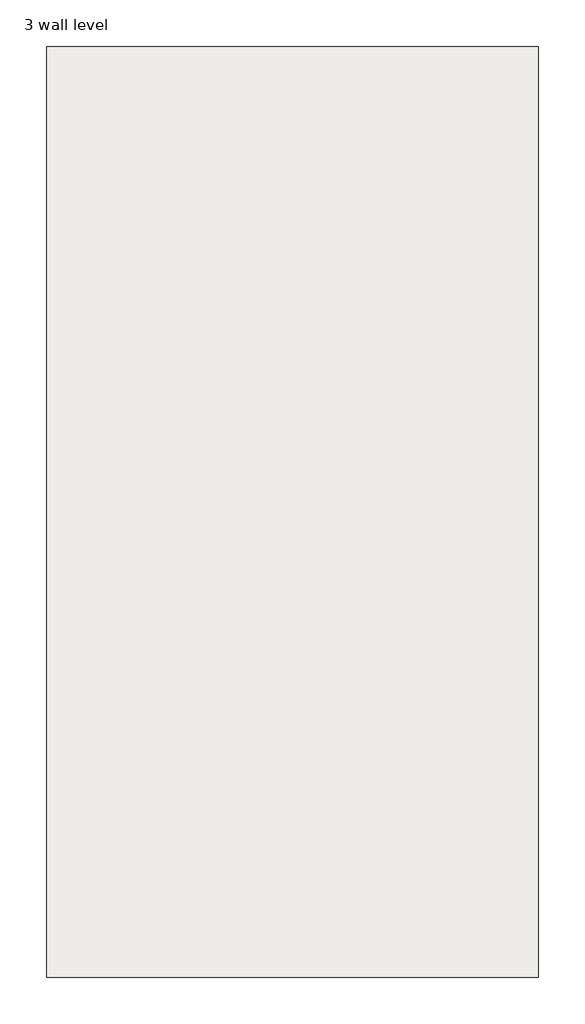
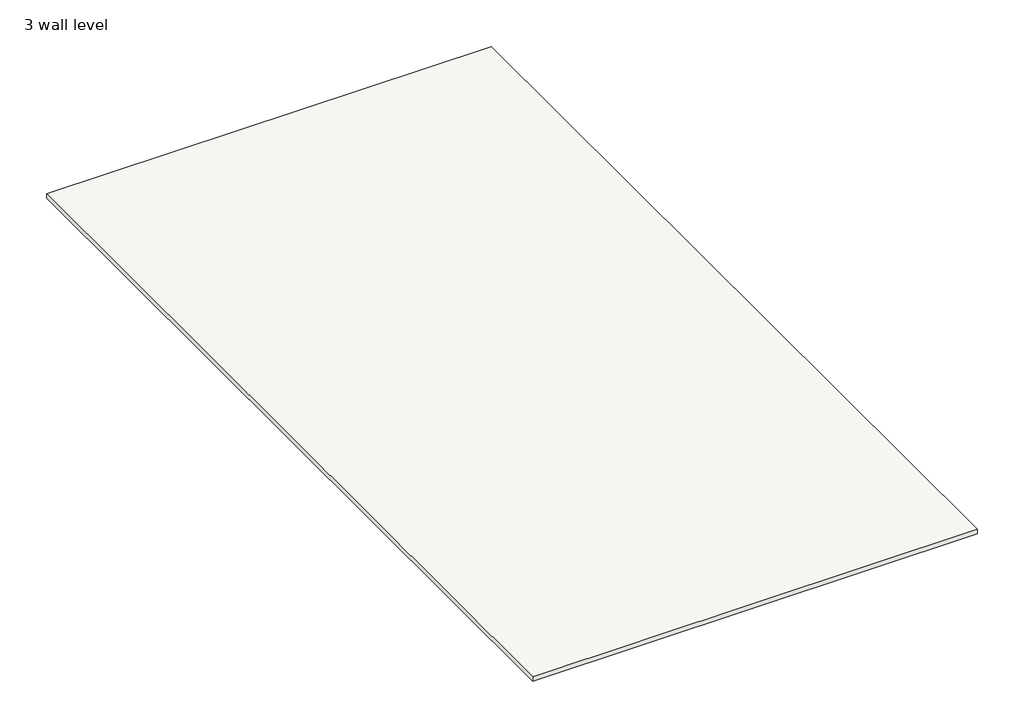
# One storey: 1 roof.
"""IFC4 building model written with IfcOpenShell, lengths in millimetres."""

from ifc_helpers import new_model, si_unit, frame, origin, place, context, project, spatial, polyline, outline, extrude, element, save

model = new_model("IFC4")

# Units and contexts
model_context = context("Model", 3, world=origin())
ifc_project = project(units=[si_unit("LENGTHUNIT", "METRE", prefix="MILLI")], contexts=[model_context])

# Site, building, storey
site = spatial("IfcSite", under=ifc_project)
building = spatial("IfcBuilding", under=site)
storey = spatial("IfcBuildingStorey", under=building, Name="3 wall level", Elevation=3505.2)

# Roof
placement = place(None, origin())
element("IfcRoof", 1, ObjectType="6\"", at=placement, inside=storey, context=model_context, shape_type="SweptSolid", body=[
    extrude(outline(polyline([(-8352.8775468, 14021.2195551), (5820.3224532, 14021.2195551), (5820.3224532, -12801.1804449), (-8352.8775468, -12801.1804449), (-8352.8775468, 14021.2195551)])), frame((0.0, 0.0, 3505.2), z_axis=(0.0, 0.0, 1.0), x_axis=(1.0, 0.0, 0.0)), (0.0, 0.0, 1.0), 152.4),
])

save(model, "model.ifc")

# Revit data of these elements
# Type "6\""
#   Assembly Code = "B1020"
#   Layers, outside or top first: 0' - 6" no material (function 1)
# Element 1 (IfcRoof, "6\"")
#   built-in parameter 1001705 = 12 (stored number, unit not read)
#   built-in parameter 1001710 = 33615
#   Phase Created = New Construction
#   Materials on its faces: "Default Roof"
# Materials
#   "Default Roof": colour RGB 88 101 114, transparency 0, Cost = 0
